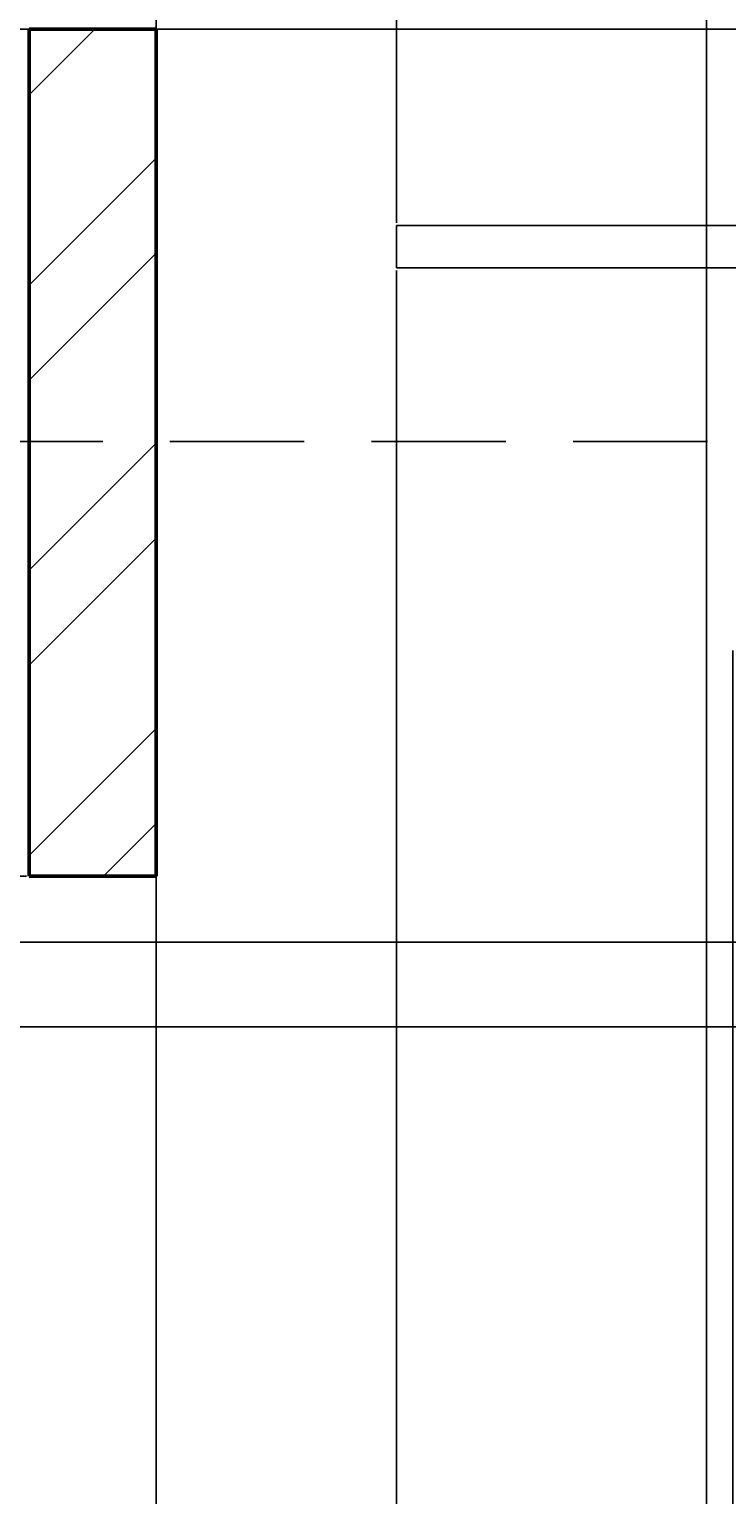
# Model space of a CAD drawing. Units: inches. Extents: x 2812 to 3051, y 1398 to 1659.
# Tile 16 of 65: x 2880 to 2897, y 1437 to 1472. Entities that reach past the tile are written whole.
import ezdxf

# ---------------------------------------------------------------- set-up
doc = ezdxf.new("R2010")
doc.units = ezdxf.units.IN
doc.linetypes.add('HIDDEN2', pattern=[4.7625, 3.175, -1.5875])
for name, color, linetype, lineweight in [('A-ANNO-DIMS', 2, 'Continuous', 18), ('S-CONC', 7, 'Continuous', 50), ('S-CONC-HIDN', 8, 'HIDDEN2', 25), ('S-CONC-PATT', 8, 'Continuous', 18), ('S-STEP', 3, 'Continuous', 25)]:
    doc.layers.add(name, color=color, linetype=linetype, lineweight=lineweight)
doc.styles.get("Standard").update_dxf_attribs({"font": 'arial.ttf'})
doc.dimstyles.get("Standard").update_dxf_attribs({"dimtxt": 0.18, "dimasz": 0.18, "dimexe": 0.18, "dimexo": 0.0625, "dimgap": 0.09, "dimtad": 0, "dimtih": 1, "dimtoh": 1, "dimdec": 4, "dimzin": 0, "dimdsep": 46, "dimtxsty": 'Standard', "dimcen": 0.09, "dimadec": 0, "dimazin": 0, "dimtfac": 1, "dimtdec": 4, "dimtofl": 0, "dimtmove": 0, "dimatfit": 3, "dimfxl": 1, "dimtolj": 1, "dimtzin": 0, "dimarcsym": 0})

# ---------------------------------------------------------------- blocks, each defined once
blk = doc.blocks.new('STEP-IRON-5')
for p, q in [((9, 1), (0, 1)), ((0, 1), (0, 0)), ((9, 0), (9, 1)), ((0, 0), (9, 0))]:
    blk.add_line(p, q)
blk = doc.blocks.new('*D29')
at = {"layer": 'A-ANNO-DIMS', "color": 0, "lineweight": -2, "transparency": 16777216}
for p, q in [((2910.742, 1598.757), (2910.742, 1397.505)), ((2883.385, 1559.757), (2883.385, 1397.505)), ((2883.565, 1397.685), (2896.598, 1397.685)), ((2910.562, 1397.685), (2897.528, 1397.685))]:
    blk.add_line(p, q, dxfattribs=at)
at = {"layer": 'A-ANNO-DIMS', "color": 0, "transparency": 16777216}
for points in [[(2883.565, 1397.715), (2883.565, 1397.655), (2883.385, 1397.685)], [(2910.562, 1397.715), (2910.562, 1397.655), (2910.742, 1397.685)]]:
    blk.add_solid(points, dxfattribs=at)
at = {"layer": 'Defpoints', "color": 0, "transparency": 16777216}
for p in [(2910.742, 1598.82), (2883.385, 1559.82), (2910.742, 1397.685)]:
    blk.add_point(p, dxfattribs=at)
at = {"layer": 'A-ANNO-DIMS', "color": 0, "transparency": 16777216, "insert": (2897.063, 1397.685), "char_height": 0.18, "attachment_point": 5}
blk.add_mtext('\\A1;27.357', dxfattribs=at)
blk = doc.blocks.new('*D44')
at = {"layer": 'A-ANNO-DIMS', "color": 0, "lineweight": -2, "transparency": 16777216}
for p, q in [((2850.748, 1487.973), (2850.748, 1397.505)), ((2896.385, 1487.973), (2896.385, 1397.505)), ((2850.928, 1397.685), (2873.17, 1397.685)), ((2896.205, 1397.685), (2873.964, 1397.685))]:
    blk.add_line(p, q, dxfattribs=at)
at = {"layer": 'A-ANNO-DIMS', "color": 0, "transparency": 16777216}
for points in [[(2850.928, 1397.715), (2850.928, 1397.655), (2850.748, 1397.685)], [(2896.205, 1397.715), (2896.205, 1397.655), (2896.385, 1397.685)]]:
    blk.add_solid(points, dxfattribs=at)
at = {"layer": 'Defpoints', "color": 0, "transparency": 16777216}
for p in [(2850.748, 1488.035), (2896.385, 1488.035), (2896.385, 1397.685)]:
    blk.add_point(p, dxfattribs=at)
at = {"layer": 'A-ANNO-DIMS', "color": 0, "transparency": 16777216, "insert": (2873.567, 1397.685), "char_height": 0.18, "attachment_point": 5}
blk.add_mtext('\\A1;45.64', dxfattribs=at)
blk = doc.blocks.new('*D45')
at = {"layer": 'A-ANNO-DIMS', "color": 0, "lineweight": -2, "transparency": 16777216}
for p, q in [((2896.385, 1487.973), (2896.385, 1397.505)), ((2941.385, 1487.973), (2941.385, 1397.505)), ((2896.565, 1397.685), (2918.662, 1397.685)), ((2941.205, 1397.685), (2919.108, 1397.685))]:
    blk.add_line(p, q, dxfattribs=at)
at = {"layer": 'A-ANNO-DIMS', "color": 0, "transparency": 16777216}
for points in [[(2896.565, 1397.715), (2896.565, 1397.655), (2896.385, 1397.685)], [(2941.205, 1397.715), (2941.205, 1397.655), (2941.385, 1397.685)]]:
    blk.add_solid(points, dxfattribs=at)
at = {"layer": 'Defpoints', "color": 0, "transparency": 16777216}
for p in [(2896.385, 1488.035), (2941.385, 1488.035), (2941.385, 1397.685)]:
    blk.add_point(p, dxfattribs=at)
at = {"layer": 'A-ANNO-DIMS', "color": 0, "transparency": 16777216, "insert": (2918.885, 1397.685), "char_height": 0.18, "attachment_point": 5}
blk.add_mtext('\\A1;45', dxfattribs=at)
blk = doc.blocks.new('*D56')
at = {"layer": 'A-ANNO-DIMS', "color": 0, "lineweight": -2, "transparency": 16777216}
for p, q in [((2880.322, 1452.035), (2811.806, 1452.035)), ((2811.986, 1451.855), (2811.986, 1434.217)), ((2811.986, 1416.215), (2811.986, 1433.853)), ((2952.322, 1416.035), (2811.806, 1416.035))]:
    blk.add_line(p, q, dxfattribs=at)
at = {"layer": 'A-ANNO-DIMS', "color": 0, "transparency": 16777216}
for points in [[(2811.956, 1451.855), (2812.016, 1451.855), (2811.986, 1452.035)], [(2811.956, 1416.215), (2812.016, 1416.215), (2811.986, 1416.035)]]:
    blk.add_solid(points, dxfattribs=at)
at = {"layer": 'Defpoints', "color": 0, "transparency": 16777216}
for p in [(2811.986, 1452.035), (2880.385, 1452.035), (2952.385, 1416.035)]:
    blk.add_point(p, dxfattribs=at)
at = {"layer": 'A-ANNO-DIMS', "color": 0, "transparency": 16777216, "insert": (2811.986, 1434.035), "char_height": 0.18, "attachment_point": 5}
blk.add_mtext('\\A1;36', dxfattribs=at)
blk = doc.blocks.new('*D59')
at = {"layer": 'A-ANNO-DIMS', "color": 0, "lineweight": -2, "transparency": 16777216}
for p, q in [((2883.385, 1452.098), (2883.385, 1659.35)), ((2883.565, 1659.17), (2885.828, 1659.17)), ((2888.878, 1659.17), (2886.615, 1659.17)), ((2889.058, 1467.465), (2889.058, 1659.35))]:
    blk.add_line(p, q, dxfattribs=at)
at = {"layer": 'A-ANNO-DIMS', "color": 0, "transparency": 16777216}
for points in [[(2883.565, 1659.2), (2883.565, 1659.14), (2883.385, 1659.17)], [(2888.878, 1659.2), (2888.878, 1659.14), (2889.058, 1659.17)]]:
    blk.add_solid(points, dxfattribs=at)
at = {"layer": 'Defpoints', "color": 0, "transparency": 16777216}
for p in [(2889.058, 1659.17), (2889.058, 1467.402), (2883.385, 1452.035)]:
    blk.add_point(p, dxfattribs=at)
at = {"layer": 'A-ANNO-DIMS', "color": 0, "transparency": 16777216, "insert": (2886.221, 1659.17), "char_height": 0.18, "attachment_point": 5}
blk.add_mtext('\\A1;5.673', dxfattribs=at)
blk = doc.blocks.new('*D60')
at = {"layer": 'A-ANNO-DIMS', "color": 0, "lineweight": -2, "transparency": 16777216}
for p, q in [((2889.058, 1466.34), (2889.058, 1397.505)), ((2897.002, 1457.364), (2897.002, 1397.505)), ((2889.238, 1397.685), (2892.637, 1397.685)), ((2896.822, 1397.685), (2893.422, 1397.685))]:
    blk.add_line(p, q, dxfattribs=at)
at = {"layer": 'A-ANNO-DIMS', "color": 0, "transparency": 16777216}
for points in [[(2889.238, 1397.715), (2889.238, 1397.655), (2889.058, 1397.685)], [(2896.822, 1397.715), (2896.822, 1397.655), (2897.002, 1397.685)]]:
    blk.add_solid(points, dxfattribs=at)
at = {"layer": 'Defpoints', "color": 0, "transparency": 16777216}
for p in [(2889.058, 1466.402), (2897.002, 1457.426), (2897.002, 1397.685)]:
    blk.add_point(p, dxfattribs=at)
at = {"layer": 'A-ANNO-DIMS', "color": 0, "transparency": 16777216, "insert": (2893.03, 1397.685), "char_height": 0.18, "attachment_point": 5}
blk.add_mtext('\\A1;7.944', dxfattribs=at)
blk = doc.blocks.new('*D75')
at = {"layer": 'A-ANNO-DIMS', "color": 0, "lineweight": -2, "transparency": 16777216}
for p, q in [((2963.812, 1448.474), (2811.806, 1448.474)), ((2811.986, 1448.294), (2811.986, 1432.437)), ((2811.986, 1416.215), (2811.986, 1432.073)), ((2961.322, 1416.035), (2811.806, 1416.035))]:
    blk.add_line(p, q, dxfattribs=at)
at = {"layer": 'A-ANNO-DIMS', "color": 0, "transparency": 16777216}
for points in [[(2811.956, 1448.294), (2812.016, 1448.294), (2811.986, 1448.474)], [(2811.956, 1416.215), (2812.016, 1416.215), (2811.986, 1416.035)]]:
    blk.add_solid(points, dxfattribs=at)
at = {"layer": 'Defpoints', "color": 0, "transparency": 16777216}
for p in [(2811.986, 1448.474), (2963.874, 1448.474), (2961.385, 1416.035)]:
    blk.add_point(p, dxfattribs=at)
at = {"layer": 'A-ANNO-DIMS', "color": 0, "transparency": 16777216, "insert": (2811.986, 1432.255), "char_height": 0.18, "attachment_point": 5}
blk.add_mtext('\\A1;32.44', dxfattribs=at)
blk = doc.blocks.new('*D76')
at = {"layer": 'A-ANNO-DIMS', "color": 0, "lineweight": -2, "transparency": 16777216}
for p, q in [((2963.812, 1450.474), (2811.806, 1450.474)), ((2811.986, 1450.294), (2811.986, 1449.654)), ((2811.986, 1448.654), (2811.986, 1449.293)), ((2963.812, 1448.474), (2811.806, 1448.474))]:
    blk.add_line(p, q, dxfattribs=at)
at = {"layer": 'A-ANNO-DIMS', "color": 0, "transparency": 16777216}
for points in [[(2811.956, 1450.294), (2812.016, 1450.294), (2811.986, 1450.474)], [(2811.956, 1448.654), (2812.016, 1448.654), (2811.986, 1448.474)]]:
    blk.add_solid(points, dxfattribs=at)
at = {"layer": 'Defpoints', "color": 0, "transparency": 16777216}
for p in [(2811.986, 1450.474), (2963.874, 1450.474), (2963.874, 1448.474)]:
    blk.add_point(p, dxfattribs=at)
at = {"layer": 'A-ANNO-DIMS', "color": 0, "transparency": 16777216, "insert": (2811.986, 1449.474), "char_height": 0.18, "attachment_point": 5}
blk.add_mtext('\\A1;2', dxfattribs=at)
blk = doc.blocks.new('*D77')
at = {"layer": 'A-ANNO-DIMS', "color": 0, "lineweight": -2, "transparency": 16777216}
for p, q in [((2961.322, 1472.035), (2811.806, 1472.035)), ((2811.986, 1471.855), (2811.986, 1461.436)), ((2811.986, 1450.654), (2811.986, 1461.073)), ((2963.812, 1450.474), (2811.806, 1450.474))]:
    blk.add_line(p, q, dxfattribs=at)
at = {"layer": 'A-ANNO-DIMS', "color": 0, "transparency": 16777216}
for points in [[(2811.956, 1471.855), (2812.016, 1471.855), (2811.986, 1472.035)], [(2811.956, 1450.654), (2812.016, 1450.654), (2811.986, 1450.474)]]:
    blk.add_solid(points, dxfattribs=at)
at = {"layer": 'Defpoints', "color": 0, "transparency": 16777216}
for p in [(2811.986, 1472.035), (2961.385, 1472.035), (2963.874, 1450.474)]:
    blk.add_point(p, dxfattribs=at)
at = {"layer": 'A-ANNO-DIMS', "color": 0, "transparency": 16777216, "insert": (2811.986, 1461.255), "char_height": 0.18, "attachment_point": 5}
blk.add_mtext('\\A1;21.56', dxfattribs=at)

msp = doc.modelspace()

# ---------------------------------------------------------------- hatches: boundary and pattern name
at = {"layer": 'S-CONC-PATT'}
h = msp.add_hatch(dxfattribs=at)
h.set_pattern_fill('ANSI32', color=256, scale=0.5)
h.paths.add_polyline_path([(2883.3849, 1472.0354), (2880.3849, 1472.0354), (2880.3849, 1462.3026), (2883.3849, 1462.3026)])
h.paths.add_polyline_path([(2883.3849, 1462.3026), (2880.3849, 1462.3026), (2880.3849, 1452.0354), (2883.3849, 1452.0354)])

# ---------------------------------------------------------------- linework, layer by layer
at = {"layer": 'S-CONC'}
for p, q in [((2880.3849, 1472.0354), (2880.3849, 1452.0354)), ((2880.3849, 1472.0354), (2883.3849, 1472.0354)), ((2883.3849, 1472.0354), (2883.3849, 1452.0354)), ((2883.3849, 1452.0354), (2880.3849, 1452.0354))]:
    msp.add_line(p, q, dxfattribs=at)
at = {"layer": 'S-CONC-HIDN'}
msp.add_line((3029.7562, 1462.3026), (2835.3849, 1462.3026), dxfattribs=at)

# ---------------------------------------------------------------- block references
at = {"layer": 'S-STEP'}
msp.add_blockref('STEP-IRON-5', (2889.0578, 1466.402), dxfattribs=at)

# ---------------------------------------------------------------- dimensions: what is measured, and where the dimension line sits
at = {"layer": 'A-ANNO-DIMS'}
for base, p1, p2, override, picture, middle in [((2889.0577, 1659.17), (2883.3849, 1452.0354), (2889.0577, 1467.4024), {"dimdec": 3, "dimlfac": 1, "dimrnd": 0, "dimzin": 0, "dimdsep": 46, "dimlunit": 2}, '*D59', (2886.2213, 1659.17)), ((2910.7415, 1397.6854), (2883.3849, 1559.82), (2910.7415, 1598.82), {"dimdec": 3, "dimlfac": 1, "dimrnd": 0, "dimzin": 0, "dimdsep": 46, "dimlunit": 2}, '*D29', (2897.0632, 1397.6854)), ((2896.3849, 1397.6854), (2850.7485, 1488.0354), (2896.3849, 1488.0354), {"dimdec": 2, "dimlfac": 1, "dimrnd": 0, "dimzin": 0, "dimdsep": 46, "dimlunit": 2}, '*D44', (2873.5667, 1397.6854)), ((2941.3849, 1397.6854), (2896.3849, 1488.0354), (2941.3849, 1488.0354), {"dimdec": 0, "dimlfac": 1, "dimrnd": 0, "dimzin": 0, "dimdsep": 46, "dimlunit": 2}, '*D45', (2918.8849, 1397.6854)), ((2897.0021, 1397.6854), (2889.0577, 1466.4024), (2897.0021, 1457.4265), {"dimdec": 3, "dimlfac": 1, "dimrnd": 0, "dimzin": 0, "dimdsep": 46, "dimlunit": 2}, '*D60', (2893.0299, 1397.6854))]:
    dim = msp.add_linear_dim(base=base, p1=p1, p2=p2, dimstyle='Standard', override=override, dxfattribs=at)
    dim.commit()
    dim.dimension.update_dxf_attribs({"geometry": picture, "text_midpoint": middle})
for base, p1, p2, override, picture, middle in [((2811.9855, 1472.0354), (2963.8741, 1450.4738), (2961.3849, 1472.0354), {"dimdec": 2, "dimlfac": 1, "dimrnd": 0, "dimzin": 0, "dimdsep": 46, "dimlunit": 2}, '*D77', (2811.9855, 1461.2546)), ((2811.9855, 1452.0354), (2952.3849, 1416.0354), (2880.3849, 1452.0354), {"dimdec": 0, "dimlfac": 1, "dimrnd": 0, "dimzin": 0, "dimdsep": 46, "dimlunit": 2}, '*D56', (2811.9855, 1434.0354)), ((2811.9855, 1450.4738), (2963.8741, 1448.4738), (2963.8741, 1450.4738), {"dimdec": 0, "dimlfac": 1, "dimrnd": 0, "dimzin": 0, "dimdsep": 46, "dimlunit": 2}, '*D76', (2811.9855, 1449.4738)), ((2811.9855, 1448.4738), (2961.3849, 1416.0354), (2963.8741, 1448.4738), {"dimdec": 2, "dimlfac": 1, "dimrnd": 0, "dimzin": 0, "dimdsep": 46, "dimlunit": 2}, '*D75', (2811.9855, 1432.2546))]:
    dim = msp.add_linear_dim(base=base, p1=p1, p2=p2, angle=90, dimstyle='Standard', override=override, dxfattribs=at)
    dim.commit()
    dim.dimension.update_dxf_attribs({"geometry": picture, "text_midpoint": middle})

doc.saveas('drawing.dxf')
